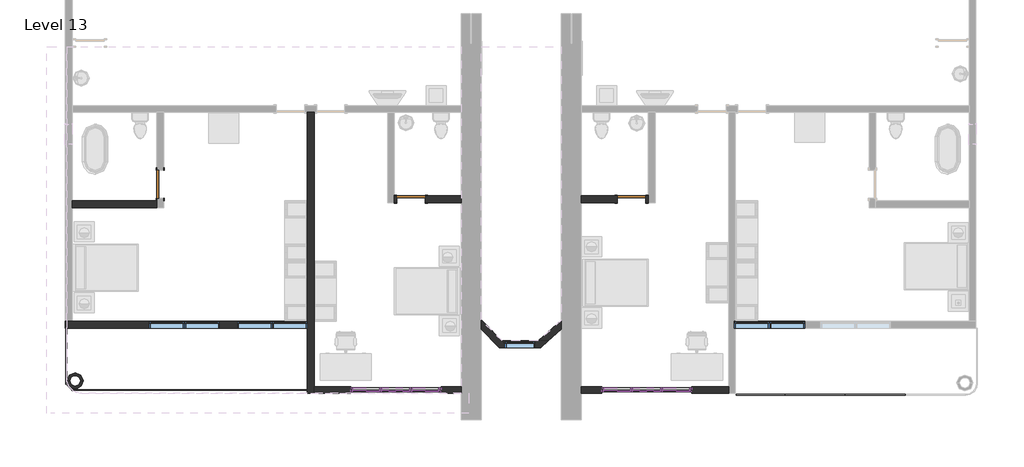
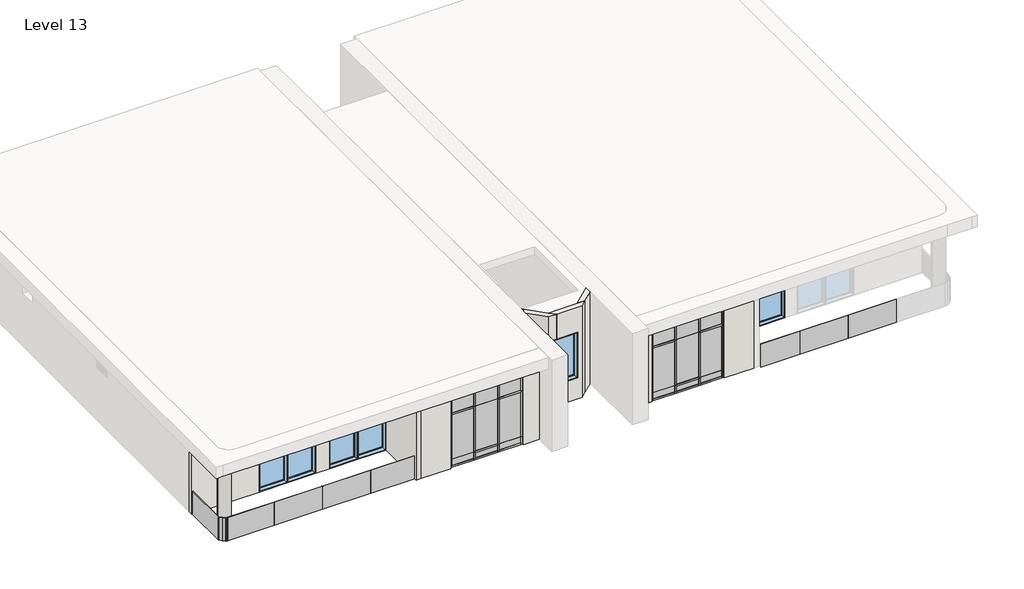
# One storey, part 1 of 3: 42 members, 30 plates, 14 walls, 7 windows, 3 doors.
"""IFC4 building model written with IfcOpenShell, lengths in millimetres."""

from ifc_helpers import new_model, si_unit, point, frame, frame_2d, origin, place, context, project, spatial, polyline, circle_curve, trimmed, segment, composite_curve, outline, extrude, faceted_brep, transform, mapped, element, save
from components import door_2703ae13, door_10fd3a06, member_c17f1be2, member_ad567e07, member_d2e7e466, member_7db1855a, member_75d1e245, member_d60e8053, member_3c3dc66a, member_2fae0574, member_410c6227, member_73c23c35, system_panel_glazed_38d54ecf, system_panel_glazed_fbb6c980, system_panel_glazed_4137532c, system_panel_glazed_6230de04, system_panel_glazed_a79f7f85, system_panel_glazed_9a5ea490, system_panel_glazed_95be5de7, system_panel_glazed_1e00a1c5, system_panel_glazed_ffe51582, system_panel_glazed_8f95e3f6, system_panel_glazed_836907cd, system_panel_glazed_688a65a2, system_panel_glazed_c1a1c740, system_panel_glazed_22bcd51f, window_9a779fa2, window_1a213a25

model = new_model("IFC4")

# Units and contexts
model_context = context("Model", 3, world=origin())
ifc_project = project(units=[si_unit("LENGTHUNIT", "METRE", prefix="MILLI")], contexts=[model_context])

# Site, building, storey
site = spatial("IfcSite", under=ifc_project)
building = spatial("IfcBuilding", under=site)
storey = spatial("IfcBuildingStorey", under=building, Name="Level 13", Elevation=43891.2)

# Doors
placement = place(None, origin())
door_shape = door_2703ae13(model_context)
element("IfcDoor", 1, ObjectType="Door-Single-Panel.0001 : 34\" x 80\"", at=placement, inside=storey, context=model_context, shape_type="MappedRepresentation", body=[
    mapped(door_shape, transform((-15765.9987704, -441.9241442, 43891.2), x_axis=(0.0, -1.0, 0.0), y_axis=(1.0, 0.0, 0.0), z_axis=(0.0, 0.0, 1.0))),
])
element("IfcDoor", 2, ObjectType="Door-Single-Panel.0001 : 34\" x 80\"", at=placement, inside=storey, context=model_context, shape_type="MappedRepresentation", body=[
    mapped(door_shape, transform((-8145.9987704, -899.1241442, 43891.2), x_axis=(-1.0, 0.0, 0.0), y_axis=(0.0, -1.0, 0.0), z_axis=(0.0, 0.0, 1.0))),
])
door_2_shape = door_10fd3a06(model_context)
element("IfcDoor", 3, ObjectType="Door-Single-Panel.0001 : 34\" x 80\"", at=placement, inside=storey, context=model_context, shape_type="MappedRepresentation", body=[
    mapped(door_2_shape, transform((-1440.3987704, -899.1241442, 43891.2), x_axis=(1.0, 0.0, 0.0), y_axis=(0.0, 1.0, 0.0), z_axis=(0.0, 0.0, 1.0))),
])

# Members
member_shape = member_c17f1be2(model_context)
element("IfcMember", 4, ObjectType="Rectangular Mullion : 2.5\" x 5\" rectangular", at=placement, inside=storey, context=model_context, shape_type="MappedRepresentation", body=[
    mapped(member_shape, transform((-9911.2987704, -6690.3241442, 46939.2), x_axis=(0.0, 0.0, 1.0), y_axis=(0.0, 1.0, 0.0), z_axis=(-1.0, 0.0, 0.0))),
])
element("IfcMember", 5, ObjectType="Rectangular Mullion : 2.5\" x 5\" rectangular", at=placement, inside=storey, context=model_context, shape_type="MappedRepresentation", body=[
    mapped(member_shape, transform((-8114.2487704, -6690.3241442, 46939.2), x_axis=(0.0, 0.0, 1.0), y_axis=(0.0, 1.0, 0.0), z_axis=(-1.0, 0.0, 0.0))),
])
element("IfcMember", 6, ObjectType="Rectangular Mullion : 2.5\" x 5\" rectangular", at=placement, inside=storey, context=model_context, shape_type="MappedRepresentation", body=[
    mapped(member_shape, transform((-2291.2987704, -6690.3241442, 46939.2), x_axis=(0.0, 0.0, 1.0), y_axis=(0.0, 1.0, 0.0), z_axis=(-1.0, 0.0, 0.0))),
])
element("IfcMember", 7, ObjectType="Rectangular Mullion : 2.5\" x 5\" rectangular", at=placement, inside=storey, context=model_context, shape_type="MappedRepresentation", body=[
    mapped(member_shape, transform((-494.2487704, -6690.3241442, 46939.2), x_axis=(0.0, 0.0, 1.0), y_axis=(0.0, 1.0, 0.0), z_axis=(-1.0, 0.0, 0.0))),
])
element("IfcMember", 8, ObjectType="Rectangular Mullion : 2.5\" x 5\" rectangular", at=placement, inside=storey, context=model_context, shape_type="MappedRepresentation", body=[
    mapped(member_shape, transform((-7295.0987704, -6690.3241442, 43891.2), x_axis=(0.0, 0.0, -1.0), y_axis=(0.0, 1.0, 0.0), z_axis=(1.0, 0.0, 0.0))),
])
element("IfcMember", 9, ObjectType="Rectangular Mullion : 2.5\" x 5\" rectangular", at=placement, inside=storey, context=model_context, shape_type="MappedRepresentation", body=[
    mapped(member_shape, transform((-9092.1487704, -6690.3241442, 43891.2), x_axis=(0.0, 0.0, -1.0), y_axis=(0.0, 1.0, 0.0), z_axis=(1.0, 0.0, 0.0))),
])
element("IfcMember", 10, ObjectType="Rectangular Mullion : 2.5\" x 5\" rectangular", at=placement, inside=storey, context=model_context, shape_type="MappedRepresentation", body=[
    mapped(member_shape, transform((324.9012296, -6690.3241442, 43891.2), x_axis=(0.0, 0.0, -1.0), y_axis=(0.0, 1.0, 0.0), z_axis=(1.0, 0.0, 0.0))),
])
element("IfcMember", 11, ObjectType="Rectangular Mullion : 2.5\" x 5\" rectangular", at=placement, inside=storey, context=model_context, shape_type="MappedRepresentation", body=[
    mapped(member_shape, transform((-1472.1487704, -6690.3241442, 43891.2), x_axis=(0.0, 0.0, -1.0), y_axis=(0.0, 1.0, 0.0), z_axis=(1.0, 0.0, 0.0))),
])
member_2_shape = member_ad567e07(model_context)
element("IfcMember", 12, ObjectType="Rectangular Mullion : 2.5\" x 5\" rectangular", at=placement, inside=storey, context=model_context, shape_type="MappedRepresentation", body=[
    mapped(member_2_shape, transform((-8114.2487704, -6690.3241442, 46024.8), x_axis=(0.0, 0.0, 1.0), y_axis=(0.0, 1.0, 0.0), z_axis=(-1.0, 0.0, 0.0))),
])
element("IfcMember", 13, ObjectType="Rectangular Mullion : 2.5\" x 5\" rectangular", at=placement, inside=storey, context=model_context, shape_type="MappedRepresentation", body=[
    mapped(member_2_shape, transform((-9911.2987704, -6690.3241442, 46024.8), x_axis=(0.0, 0.0, 1.0), y_axis=(0.0, 1.0, 0.0), z_axis=(-1.0, 0.0, 0.0))),
])
element("IfcMember", 14, ObjectType="Rectangular Mullion : 2.5\" x 5\" rectangular", at=placement, inside=storey, context=model_context, shape_type="MappedRepresentation", body=[
    mapped(member_2_shape, transform((-494.2487704, -6690.3241442, 46024.8), x_axis=(0.0, 0.0, 1.0), y_axis=(0.0, 1.0, 0.0), z_axis=(-1.0, 0.0, 0.0))),
])
element("IfcMember", 15, ObjectType="Rectangular Mullion : 2.5\" x 5\" rectangular", at=placement, inside=storey, context=model_context, shape_type="MappedRepresentation", body=[
    mapped(member_2_shape, transform((-2291.2987704, -6690.3241442, 46024.8), x_axis=(0.0, 0.0, 1.0), y_axis=(0.0, 1.0, 0.0), z_axis=(-1.0, 0.0, 0.0))),
])
member_3_shape = member_d2e7e466(model_context)
element("IfcMember", 16, ObjectType="Rectangular Mullion : 2.5\" x 5\" rectangular", at=placement, inside=storey, context=model_context, shape_type="MappedRepresentation", body=[
    mapped(member_3_shape, transform((-8177.7487704, -6690.3241442, 43891.2), x_axis=(0.0, 0.0, -1.0), y_axis=(0.0, 1.0, 0.0), z_axis=(1.0, 0.0, 0.0))),
])
element("IfcMember", 17, ObjectType="Rectangular Mullion : 2.5\" x 5\" rectangular", at=placement, inside=storey, context=model_context, shape_type="MappedRepresentation", body=[
    mapped(member_3_shape, transform((-557.7487704, -6690.3241442, 43891.2), x_axis=(0.0, 0.0, -1.0), y_axis=(0.0, 1.0, 0.0), z_axis=(1.0, 0.0, 0.0))),
])
member_4_shape = member_7db1855a(model_context)
element("IfcMember", 18, ObjectType="Rectangular Mullion : 2.5\" x 5\" rectangular", at=placement, inside=storey, context=model_context, shape_type="MappedRepresentation", body=[
    mapped(member_4_shape, transform((-9028.6487704, -6690.3241442, 44196.0), x_axis=(0.0, 0.0, 1.0), y_axis=(0.0, 1.0, 0.0), z_axis=(-1.0, 0.0, 0.0))),
])
element("IfcMember", 19, ObjectType="Rectangular Mullion : 2.5\" x 5\" rectangular", at=placement, inside=storey, context=model_context, shape_type="MappedRepresentation", body=[
    mapped(member_4_shape, transform((-1408.6487704, -6690.3241442, 44196.0), x_axis=(0.0, 0.0, 1.0), y_axis=(0.0, 1.0, 0.0), z_axis=(-1.0, 0.0, 0.0))),
])
element("IfcMember", 20, ObjectType="Rectangular Mullion : 2.5\" x 5\" rectangular", at=placement, inside=storey, context=model_context, shape_type="MappedRepresentation", body=[
    mapped(member_3_shape, transform((-9028.6487704, -6690.3241442, 46939.2), x_axis=(0.0, 0.0, 1.0), y_axis=(0.0, 1.0, 0.0), z_axis=(-1.0, 0.0, 0.0))),
])
element("IfcMember", 21, ObjectType="Rectangular Mullion : 2.5\" x 5\" rectangular", at=placement, inside=storey, context=model_context, shape_type="MappedRepresentation", body=[
    mapped(member_3_shape, transform((-1408.6487704, -6690.3241442, 46939.2), x_axis=(0.0, 0.0, 1.0), y_axis=(0.0, 1.0, 0.0), z_axis=(-1.0, 0.0, 0.0))),
])
member_5_shape = member_75d1e245(model_context)
element("IfcMember", 22, ObjectType="Rectangular Mullion : 2.5\" x 5\" rectangular", at=placement, inside=storey, context=model_context, shape_type="MappedRepresentation", body=[
    mapped(member_5_shape, transform((-8145.9987704, -6690.3241442, 43891.2), x_axis=(-1.0, 0.0, 0.0), y_axis=(0.0, 1.0, 0.0), z_axis=(0.0, 0.0, -1.0))),
])
element("IfcMember", 23, ObjectType="Rectangular Mullion : 2.5\" x 5\" rectangular", at=placement, inside=storey, context=model_context, shape_type="MappedRepresentation", body=[
    mapped(member_5_shape, transform((-9060.3987704, -6690.3241442, 43891.2), x_axis=(-1.0, 0.0, 0.0), y_axis=(0.0, 1.0, 0.0), z_axis=(0.0, 0.0, -1.0))),
])
element("IfcMember", 24, ObjectType="Rectangular Mullion : 2.5\" x 5\" rectangular", at=placement, inside=storey, context=model_context, shape_type="MappedRepresentation", body=[
    mapped(member_5_shape, transform((-525.9987704, -6690.3241442, 43891.2), x_axis=(-1.0, 0.0, 0.0), y_axis=(0.0, 1.0, 0.0), z_axis=(0.0, 0.0, -1.0))),
])
element("IfcMember", 25, ObjectType="Rectangular Mullion : 2.5\" x 5\" rectangular", at=placement, inside=storey, context=model_context, shape_type="MappedRepresentation", body=[
    mapped(member_5_shape, transform((-1440.3987704, -6690.3241442, 43891.2), x_axis=(-1.0, 0.0, 0.0), y_axis=(0.0, 1.0, 0.0), z_axis=(0.0, 0.0, -1.0))),
])
member_6_shape = member_d60e8053(model_context)
element("IfcMember", 26, ObjectType="Rectangular Mullion : 2.5\" x 5\" rectangular", at=placement, inside=storey, context=model_context, shape_type="MappedRepresentation", body=[
    mapped(member_6_shape, transform((-8145.9987704, -6690.3241442, 44196.0), x_axis=(-1.0, 0.0, 0.0), y_axis=(0.0, 1.0, 0.0), z_axis=(0.0, 0.0, -1.0))),
])
element("IfcMember", 27, ObjectType="Rectangular Mullion : 2.5\" x 5\" rectangular", at=placement, inside=storey, context=model_context, shape_type="MappedRepresentation", body=[
    mapped(member_6_shape, transform((-9060.3987704, -6690.3241442, 44196.0), x_axis=(-1.0, 0.0, 0.0), y_axis=(0.0, 1.0, 0.0), z_axis=(0.0, 0.0, -1.0))),
])
element("IfcMember", 28, ObjectType="Rectangular Mullion : 2.5\" x 5\" rectangular", at=placement, inside=storey, context=model_context, shape_type="MappedRepresentation", body=[
    mapped(member_6_shape, transform((-525.9987704, -6690.3241442, 44196.0), x_axis=(-1.0, 0.0, 0.0), y_axis=(0.0, 1.0, 0.0), z_axis=(0.0, 0.0, -1.0))),
])
element("IfcMember", 29, ObjectType="Rectangular Mullion : 2.5\" x 5\" rectangular", at=placement, inside=storey, context=model_context, shape_type="MappedRepresentation", body=[
    mapped(member_6_shape, transform((-1440.3987704, -6690.3241442, 44196.0), x_axis=(-1.0, 0.0, 0.0), y_axis=(0.0, 1.0, 0.0), z_axis=(0.0, 0.0, -1.0))),
])
member_7_shape = member_3c3dc66a(model_context)
element("IfcMember", 30, ObjectType="Rectangular Mullion : 2.5\" x 5\" rectangular", at=placement, inside=storey, context=model_context, shape_type="MappedRepresentation", body=[
    mapped(member_7_shape, transform((-9974.7987704, -6690.3241442, 43891.2), x_axis=(-1.0, 0.0, 0.0), y_axis=(0.0, 1.0, 0.0), z_axis=(0.0, 0.0, -1.0))),
])
element("IfcMember", 31, ObjectType="Rectangular Mullion : 2.5\" x 5\" rectangular", at=placement, inside=storey, context=model_context, shape_type="MappedRepresentation", body=[
    mapped(member_7_shape, transform((-2354.7987704, -6690.3241442, 43891.2), x_axis=(-1.0, 0.0, 0.0), y_axis=(0.0, 1.0, 0.0), z_axis=(0.0, 0.0, -1.0))),
])
member_8_shape = member_2fae0574(model_context)
element("IfcMember", 32, ObjectType="Rectangular Mullion : 2.5\" x 5\" rectangular", at=placement, inside=storey, context=model_context, shape_type="MappedRepresentation", body=[
    mapped(member_8_shape, transform((-9974.7987704, -6690.3241442, 44196.0), x_axis=(-1.0, 0.0, 0.0), y_axis=(0.0, 1.0, 0.0), z_axis=(0.0, 0.0, -1.0))),
])
element("IfcMember", 33, ObjectType="Rectangular Mullion : 2.5\" x 5\" rectangular", at=placement, inside=storey, context=model_context, shape_type="MappedRepresentation", body=[
    mapped(member_8_shape, transform((-2354.7987704, -6690.3241442, 44196.0), x_axis=(-1.0, 0.0, 0.0), y_axis=(0.0, 1.0, 0.0), z_axis=(0.0, 0.0, -1.0))),
])
element("IfcMember", 34, ObjectType="Rectangular Mullion : 2.5\" x 5\" rectangular", at=placement, inside=storey, context=model_context, shape_type="MappedRepresentation", body=[
    mapped(member_8_shape, transform((-7231.5987704, -6690.3241442, 46024.8), x_axis=(1.0, 0.0, 0.0), y_axis=(0.0, 1.0, 0.0), z_axis=(0.0, 0.0, 1.0))),
])
element("IfcMember", 35, ObjectType="Rectangular Mullion : 2.5\" x 5\" rectangular", at=placement, inside=storey, context=model_context, shape_type="MappedRepresentation", body=[
    mapped(member_8_shape, transform((388.4012296, -6690.3241442, 46024.8), x_axis=(1.0, 0.0, 0.0), y_axis=(0.0, 1.0, 0.0), z_axis=(0.0, 0.0, 1.0))),
])
element("IfcMember", 36, ObjectType="Rectangular Mullion : 2.5\" x 5\" rectangular", at=placement, inside=storey, context=model_context, shape_type="MappedRepresentation", body=[
    mapped(member_7_shape, transform((-7231.5987704, -6690.3241442, 44196.0), x_axis=(1.0, 0.0, 0.0), y_axis=(0.0, 1.0, 0.0), z_axis=(0.0, 0.0, 1.0))),
])
element("IfcMember", 37, ObjectType="Rectangular Mullion : 2.5\" x 5\" rectangular", at=placement, inside=storey, context=model_context, shape_type="MappedRepresentation", body=[
    mapped(member_7_shape, transform((388.4012296, -6690.3241442, 44196.0), x_axis=(1.0, 0.0, 0.0), y_axis=(0.0, 1.0, 0.0), z_axis=(0.0, 0.0, 1.0))),
])
member_9_shape = member_410c6227(model_context)
element("IfcMember", 38, ObjectType="Rectangular Mullion : 2.5\" x 5\" rectangular", at=placement, inside=storey, context=model_context, shape_type="MappedRepresentation", body=[
    mapped(member_9_shape, transform((-8145.9987704, -6690.3241442, 46024.8), x_axis=(-1.0, 0.0, 0.0), y_axis=(0.0, 1.0, 0.0), z_axis=(0.0, 0.0, -1.0))),
])
element("IfcMember", 39, ObjectType="Rectangular Mullion : 2.5\" x 5\" rectangular", at=placement, inside=storey, context=model_context, shape_type="MappedRepresentation", body=[
    mapped(member_9_shape, transform((-9060.3987704, -6690.3241442, 46024.8), x_axis=(-1.0, 0.0, 0.0), y_axis=(0.0, 1.0, 0.0), z_axis=(0.0, 0.0, -1.0))),
])
element("IfcMember", 40, ObjectType="Rectangular Mullion : 2.5\" x 5\" rectangular", at=placement, inside=storey, context=model_context, shape_type="MappedRepresentation", body=[
    mapped(member_9_shape, transform((-525.9987704, -6690.3241442, 46024.8), x_axis=(-1.0, 0.0, 0.0), y_axis=(0.0, 1.0, 0.0), z_axis=(0.0, 0.0, -1.0))),
])
element("IfcMember", 41, ObjectType="Rectangular Mullion : 2.5\" x 5\" rectangular", at=placement, inside=storey, context=model_context, shape_type="MappedRepresentation", body=[
    mapped(member_9_shape, transform((-1440.3987704, -6690.3241442, 46024.8), x_axis=(-1.0, 0.0, 0.0), y_axis=(0.0, 1.0, 0.0), z_axis=(0.0, 0.0, -1.0))),
])
member_10_shape = member_73c23c35(model_context)
element("IfcMember", 42, ObjectType="Rectangular Mullion : 2.5\" x 5\" rectangular", at=placement, inside=storey, context=model_context, shape_type="MappedRepresentation", body=[
    mapped(member_10_shape, transform((-7231.5987704, -6690.3241442, 46939.2), x_axis=(1.0, 0.0, 0.0), y_axis=(0.0, 1.0, 0.0), z_axis=(0.0, 0.0, 1.0))),
])
element("IfcMember", 43, ObjectType="Rectangular Mullion : 2.5\" x 5\" rectangular", at=placement, inside=storey, context=model_context, shape_type="MappedRepresentation", body=[
    mapped(member_10_shape, transform((388.4012296, -6690.3241442, 46939.2), x_axis=(1.0, 0.0, 0.0), y_axis=(0.0, 1.0, 0.0), z_axis=(0.0, 0.0, 1.0))),
])
element("IfcMember", 44, ObjectType="Rectangular Mullion : 2.5\" x 5\" rectangular", at=placement, inside=storey, context=model_context, shape_type="MappedRepresentation", body=[
    mapped(member_10_shape, transform((-9974.7987704, -6690.3241442, 46024.8), x_axis=(-1.0, 0.0, 0.0), y_axis=(0.0, 1.0, 0.0), z_axis=(0.0, 0.0, -1.0))),
])
element("IfcMember", 45, ObjectType="Rectangular Mullion : 2.5\" x 5\" rectangular", at=placement, inside=storey, context=model_context, shape_type="MappedRepresentation", body=[
    mapped(member_10_shape, transform((-2354.7987704, -6690.3241442, 46024.8), x_axis=(-1.0, 0.0, 0.0), y_axis=(0.0, 1.0, 0.0), z_axis=(0.0, 0.0, -1.0))),
])

# Plates
system_panel_glazed_shape = system_panel_glazed_38d54ecf(model_context)
element("IfcPlate", 46, ObjectType="System Panel : Glazed", at=placement, inside=storey, context=model_context, shape_type="MappedRepresentation", body=[
    mapped(system_panel_glazed_shape, transform((-8603.1987704, -6690.3241442, 44227.75), x_axis=(-1.0, 0.0, 0.0), y_axis=(0.0, -1.0, 0.0), z_axis=(0.0, 0.0, 1.0))),
])
element("IfcPlate", 47, ObjectType="System Panel : Glazed", at=placement, inside=storey, context=model_context, shape_type="MappedRepresentation", body=[
    mapped(system_panel_glazed_shape, transform((-983.1987704, -6690.3241442, 44227.75), x_axis=(-1.0, 0.0, 0.0), y_axis=(0.0, -1.0, 0.0), z_axis=(0.0, 0.0, 1.0))),
])
system_panel_glazed_2_shape = system_panel_glazed_fbb6c980(model_context)
element("IfcPlate", 48, ObjectType="System Panel : Glazed", at=placement, inside=storey, context=model_context, shape_type="MappedRepresentation", body=[
    mapped(system_panel_glazed_2_shape, transform((-8603.1987704, -6690.3241442, 43954.7), x_axis=(-1.0, 0.0, 0.0), y_axis=(0.0, -1.0, 0.0), z_axis=(0.0, 0.0, 1.0))),
])
element("IfcPlate", 49, ObjectType="System Panel : Glazed", at=placement, inside=storey, context=model_context, shape_type="MappedRepresentation", body=[
    mapped(system_panel_glazed_2_shape, transform((-983.1987704, -6690.3241442, 43954.7), x_axis=(-1.0, 0.0, 0.0), y_axis=(0.0, -1.0, 0.0), z_axis=(0.0, 0.0, 1.0))),
])
system_panel_glazed_3_shape = system_panel_glazed_4137532c(model_context)
element("IfcPlate", 50, ObjectType="System Panel : Glazed", at=placement, inside=storey, context=model_context, shape_type="MappedRepresentation", body=[
    mapped(system_panel_glazed_3_shape, transform((-7704.6737704, -6690.3241442, 43954.7), x_axis=(-1.0, 0.0, 0.0), y_axis=(0.0, -1.0, 0.0), z_axis=(0.0, 0.0, 1.0))),
])
element("IfcPlate", 51, ObjectType="System Panel : Glazed", at=placement, inside=storey, context=model_context, shape_type="MappedRepresentation", body=[
    mapped(system_panel_glazed_3_shape, transform((-9501.7237704, -6690.3241442, 43954.7), x_axis=(-1.0, 0.0, 0.0), y_axis=(0.0, -1.0, 0.0), z_axis=(0.0, 0.0, 1.0))),
])
element("IfcPlate", 52, ObjectType="System Panel : Glazed", at=placement, inside=storey, context=model_context, shape_type="MappedRepresentation", body=[
    mapped(system_panel_glazed_3_shape, transform((-84.6737704, -6690.3241442, 43954.7), x_axis=(-1.0, 0.0, 0.0), y_axis=(0.0, -1.0, 0.0), z_axis=(0.0, 0.0, 1.0))),
])
element("IfcPlate", 53, ObjectType="System Panel : Glazed", at=placement, inside=storey, context=model_context, shape_type="MappedRepresentation", body=[
    mapped(system_panel_glazed_3_shape, transform((-1881.7237704, -6690.3241442, 43954.7), x_axis=(-1.0, 0.0, 0.0), y_axis=(0.0, -1.0, 0.0), z_axis=(0.0, 0.0, 1.0))),
])
system_panel_glazed_4_shape = system_panel_glazed_6230de04(model_context)
element("IfcPlate", 54, ObjectType="System Panel : Glazed", at=placement, inside=storey, context=model_context, shape_type="MappedRepresentation", body=[
    mapped(system_panel_glazed_4_shape, transform((-7704.6737704, -6690.3241442, 44196.0), x_axis=(-1.0, 0.0, 0.0), y_axis=(0.0, -1.0, 0.0), z_axis=(0.0, 0.0, 1.0))),
])
element("IfcPlate", 55, ObjectType="System Panel : Glazed", at=placement, inside=storey, context=model_context, shape_type="MappedRepresentation", body=[
    mapped(system_panel_glazed_4_shape, transform((-9501.7237704, -6690.3241442, 44196.0), x_axis=(-1.0, 0.0, 0.0), y_axis=(0.0, -1.0, 0.0), z_axis=(0.0, 0.0, 1.0))),
])
element("IfcPlate", 56, ObjectType="System Panel : Glazed", at=placement, inside=storey, context=model_context, shape_type="MappedRepresentation", body=[
    mapped(system_panel_glazed_4_shape, transform((-84.6737704, -6690.3241442, 44196.0), x_axis=(-1.0, 0.0, 0.0), y_axis=(0.0, -1.0, 0.0), z_axis=(0.0, 0.0, 1.0))),
])
element("IfcPlate", 57, ObjectType="System Panel : Glazed", at=placement, inside=storey, context=model_context, shape_type="MappedRepresentation", body=[
    mapped(system_panel_glazed_4_shape, transform((-1881.7237704, -6690.3241442, 44196.0), x_axis=(-1.0, 0.0, 0.0), y_axis=(0.0, -1.0, 0.0), z_axis=(0.0, 0.0, 1.0))),
])
system_panel_glazed_5_shape = system_panel_glazed_a79f7f85(model_context)
element("IfcPlate", 58, ObjectType="System Panel : Glazed", at=placement, inside=storey, context=model_context, shape_type="MappedRepresentation", body=[
    mapped(system_panel_glazed_5_shape, transform((-7704.6737704, -6690.3241442, 46056.55), x_axis=(-1.0, 0.0, 0.0), y_axis=(0.0, -1.0, 0.0), z_axis=(0.0, 0.0, 1.0))),
])
element("IfcPlate", 59, ObjectType="System Panel : Glazed", at=placement, inside=storey, context=model_context, shape_type="MappedRepresentation", body=[
    mapped(system_panel_glazed_5_shape, transform((-9501.7237704, -6690.3241442, 46056.55), x_axis=(-1.0, 0.0, 0.0), y_axis=(0.0, -1.0, 0.0), z_axis=(0.0, 0.0, 1.0))),
])
element("IfcPlate", 60, ObjectType="System Panel : Glazed", at=placement, inside=storey, context=model_context, shape_type="MappedRepresentation", body=[
    mapped(system_panel_glazed_5_shape, transform((-84.6737704, -6690.3241442, 46056.55), x_axis=(-1.0, 0.0, 0.0), y_axis=(0.0, -1.0, 0.0), z_axis=(0.0, 0.0, 1.0))),
])
element("IfcPlate", 61, ObjectType="System Panel : Glazed", at=placement, inside=storey, context=model_context, shape_type="MappedRepresentation", body=[
    mapped(system_panel_glazed_5_shape, transform((-1881.7237704, -6690.3241442, 46056.55), x_axis=(-1.0, 0.0, 0.0), y_axis=(0.0, -1.0, 0.0), z_axis=(0.0, 0.0, 1.0))),
])
system_panel_glazed_6_shape = system_panel_glazed_9a5ea490(model_context)
element("IfcPlate", 62, ObjectType="System Panel : Glazed", at=placement, inside=storey, context=model_context, shape_type="MappedRepresentation", body=[
    mapped(system_panel_glazed_6_shape, transform((-8603.1987704, -6690.3241442, 46024.8), x_axis=(-1.0, 0.0, 0.0), y_axis=(0.0, -1.0, 0.0), z_axis=(0.0, 0.0, 1.0))),
])
element("IfcPlate", 63, ObjectType="System Panel : Glazed", at=placement, inside=storey, context=model_context, shape_type="MappedRepresentation", body=[
    mapped(system_panel_glazed_6_shape, transform((-983.1987704, -6690.3241442, 46024.8), x_axis=(-1.0, 0.0, 0.0), y_axis=(0.0, -1.0, 0.0), z_axis=(0.0, 0.0, 1.0))),
])
system_panel_glazed_7_shape = system_panel_glazed_95be5de7(model_context)
element("IfcPlate", 64, ObjectType="System Panel : Glazed", at=placement, inside=storey, context=model_context, shape_type="MappedRepresentation", body=[
    mapped(system_panel_glazed_7_shape, transform((-15707.2305745, -6723.6923401, 43891.2), x_axis=(1.0, 0.0, 0.0), y_axis=(0.0, 1.0, 0.0), z_axis=(0.0, 0.0, 1.0))),
])
element("IfcPlate", 65, ObjectType="System Panel : Glazed", at=placement, inside=storey, context=model_context, shape_type="MappedRepresentation", body=[
    mapped(system_panel_glazed_7_shape, transform((-13878.4305745, -6723.6923401, 43891.2), x_axis=(1.0, 0.0, 0.0), y_axis=(0.0, 1.0, 0.0), z_axis=(0.0, 0.0, 1.0))),
])
element("IfcPlate", 66, ObjectType="System Panel : Glazed", at=placement, inside=storey, context=model_context, shape_type="MappedRepresentation", body=[
    mapped(system_panel_glazed_7_shape, transform((5957.9120092, -6810.4133646, 43891.2), x_axis=(-1.0, 0.0, 0.0), y_axis=(0.0, -1.0, 0.0), z_axis=(0.0, 0.0, 1.0))),
])
element("IfcPlate", 67, ObjectType="System Panel : Glazed", at=placement, inside=storey, context=model_context, shape_type="MappedRepresentation", body=[
    mapped(system_panel_glazed_7_shape, transform((4129.1120092, -6810.4133646, 43891.2), x_axis=(-1.0, 0.0, 0.0), y_axis=(0.0, -1.0, 0.0), z_axis=(0.0, 0.0, 1.0))),
])
system_panel_glazed_8_shape = system_panel_glazed_1e00a1c5(model_context)
element("IfcPlate", 68, ObjectType="System Panel : Glazed", at=placement, inside=storey, context=model_context, shape_type="MappedRepresentation", body=[
    mapped(system_panel_glazed_8_shape, transform((2478.1120092, -6810.4133646, 43891.2), x_axis=(-1.0, 0.0, 0.0), y_axis=(0.0, -1.0, 0.0), z_axis=(0.0, 0.0, 1.0))),
])
system_panel_glazed_9_shape = system_panel_glazed_ffe51582(model_context)
element("IfcPlate", 69, ObjectType="System Panel : Glazed", at=placement, inside=storey, context=model_context, shape_type="MappedRepresentation", body=[
    mapped(system_panel_glazed_9_shape, transform((-18451.9713429, -6722.1515718, 43891.2), x_axis=(0.7071067811865462, -0.7071067811865488, 0.0), y_axis=(0.7071067811865488, 0.7071067811865462, 0.0), z_axis=(0.0, 0.0, 1.0))),
])
system_panel_glazed_10_shape = system_panel_glazed_8f95e3f6(model_context)
element("IfcPlate", 70, ObjectType="System Panel : Glazed", at=placement, inside=storey, context=model_context, shape_type="MappedRepresentation", body=[
    mapped(system_panel_glazed_10_shape, transform((-18648.8987704, -5667.9741442, 43891.2), x_axis=(0.0, -1.0, 0.0), y_axis=(1.0, 0.0, 0.0), z_axis=(0.0, 0.0, 1.0))),
])
system_panel_glazed_11_shape = system_panel_glazed_836907cd(model_context)
element("IfcPlate", 71, ObjectType="System Panel : Glazed", at=placement, inside=storey, context=model_context, shape_type="MappedRepresentation", body=[
    mapped(system_panel_glazed_11_shape, transform((-18418.6805745, -6723.6923401, 43891.2), x_axis=(1.0, 0.0, 0.0), y_axis=(0.0, 1.0, 0.0), z_axis=(0.0, 0.0, 1.0))),
])
system_panel_glazed_12_shape = system_panel_glazed_688a65a2(model_context)
element("IfcPlate", 72, ObjectType="System Panel : Glazed", at=placement, inside=storey, context=model_context, shape_type="MappedRepresentation", body=[
    mapped(system_panel_glazed_12_shape, transform((-12129.8146725, -6723.6923401, 43891.2), x_axis=(1.0, 0.0, 0.0), y_axis=(0.0, 1.0, 0.0), z_axis=(0.0, 0.0, 1.0))),
])
system_panel_glazed_13_shape = system_panel_glazed_c1a1c740(model_context)
element("IfcPlate", 73, ObjectType="System Panel : Glazed", at=placement, inside=storey, context=model_context, shape_type="MappedRepresentation", body=[
    mapped(system_panel_glazed_13_shape, transform((-17504.2805745, -6723.6923401, 43891.2), x_axis=(1.0, 0.0, 0.0), y_axis=(0.0, 1.0, 0.0), z_axis=(0.0, 0.0, 1.0))),
])
system_panel_glazed_14_shape = system_panel_glazed_22bcd51f(model_context)
element("IfcPlate", 74, ObjectType="System Panel : Glazed", at=placement, inside=storey, context=model_context, shape_type="MappedRepresentation", body=[
    mapped(system_panel_glazed_14_shape, transform((-18600.0521056, -6574.070809, 43891.2), x_axis=(0.7071067811865462, -0.7071067811865488, 0.0), y_axis=(0.7071067811865488, 0.7071067811865462, 0.0), z_axis=(0.0, 0.0, 1.0))),
])
element("IfcPlate", 75, ObjectType="System Panel : Glazed", at=placement, inside=storey, context=model_context, shape_type="MappedRepresentation", body=[
    mapped(system_panel_glazed_14_shape, transform((-18502.3587761, -6671.7641386, 43891.2), x_axis=(0.7071067811865462, -0.7071067811865488, 0.0), y_axis=(0.7071067811865488, 0.7071067811865462, 0.0), z_axis=(0.0, 0.0, 1.0))),
])

# Walls
element("IfcWall", 76, ObjectType="Generic - 3\" green 2", at=placement, inside=storey, context=model_context, shape_type="SweptSolid", body=[
    extrude(outline(composite_curve([segment(polyline([(-18518.7237704, -6418.8616442), (-18594.9237704, -6418.8616442)]), True, "CONTINUOUS"), segment(trimmed(circle_curve(frame_2d((-18353.6237704, -6418.8616442)), 241.3), [point((-18594.9237704, -6418.8616442))], [point((-18112.3237704, -6418.8616442))], False, "CARTESIAN"), True, "CONTINUOUS"), segment(polyline([(-18112.3237704, -6418.8616442), (-18188.5237704, -6418.8616442)]), True, "CONTINUOUS"), segment(trimmed(circle_curve(frame_2d((-18353.6237704, -6418.8616442)), 165.1), [point((-18188.5237704, -6418.8616442))], [point((-18518.7237704, -6418.8616442))], True, "CARTESIAN"), True, "CONTINUOUS")], self_intersect=False)), frame((0.0, 0.0, 43891.2), z_axis=(0.0, 0.0, 1.0), x_axis=(1.0, 0.0, 0.0)), (0.0, 0.0, 1.0), 3048.0),
])
element("IfcWall", 77, ObjectType="Generic - 3\" green 2", at=placement, inside=storey, context=model_context, shape_type="SweptSolid", body=[
    extrude(outline(composite_curve([segment(polyline([(-18188.5237704, -6418.8616442), (-18112.3237704, -6418.8616442)]), True, "CONTINUOUS"), segment(trimmed(circle_curve(frame_2d((-18353.6237704, -6418.8616442)), 241.3), [point((-18112.3237704, -6418.8616442))], [point((-18594.9237704, -6418.8616442))], False, "CARTESIAN"), True, "CONTINUOUS"), segment(polyline([(-18594.9237704, -6418.8616442), (-18518.7237704, -6418.8616442)]), True, "CONTINUOUS"), segment(trimmed(circle_curve(frame_2d((-18353.6237704, -6418.8616442)), 165.1), [point((-18518.7237704, -6418.8616442))], [point((-18188.5237704, -6418.8616442))], True, "CARTESIAN"), True, "CONTINUOUS")], self_intersect=False)), frame((0.0, 0.0, 43891.2), z_axis=(0.0, 0.0, 1.0), x_axis=(1.0, 0.0, 0.0)), (0.0, 0.0, 1.0), 3048.0),
])
element("IfcWall", 78, ObjectType="Generic - 8\" cream", at=placement, inside=storey, context=model_context, shape_type="Brep", body=[
    faceted_brep([(-11295.5987704, 1742.4758558, 43891.2), (-11295.5987704, -6791.9241442, 43891.2), (-11295.5987704, -6791.9241442, 46939.2), (-11295.5987704, -4810.7241442, 46939.2), (-11295.5987704, -4607.5241442, 46939.2), (-11295.5987704, 1742.4758558, 46939.2), (-11092.3987704, 1742.4758558, 43891.2), (-11092.3987704, 1742.4758558, 46939.2), (-11092.3987704, -6588.7241442, 46939.2), (-11092.3987704, -6791.9241442, 46939.2), (-11092.3987704, -6791.9241442, 43891.2), (-11092.3987704, -6588.7241442, 43891.2)], [[[0, 1, 2, 3, 4, 5]], [[6, 7, 8, 9, 10, 11]], [[1, 0, 6, 11, 10]], [[5, 4, 3, 2, 9, 8, 7]], [[0, 5, 7, 6]], [[2, 1, 10, 9]]]),
])
element("IfcWall", 79, ObjectType="Generic - 8\" cream", at=placement, inside=storey, context=model_context, shape_type="SweptSolid", body=[
    extrude(outline(polyline([(-18445.6987704, -949.9241442), (-15867.5987704, -949.9241442), (-15867.5987704, -1153.1241442), (-18445.6987704, -1153.1241442), (-18445.6987704, -949.9241442)])), frame((0.0, 0.0, 43891.2), z_axis=(0.0, 0.0, 1.0), x_axis=(1.0, 0.0, 0.0)), (0.0, 0.0, 1.0), 3048.0),
])
element("IfcWall", 80, ObjectType="Generic - 8\" cream", at=placement, inside=storey, context=model_context, shape_type="SweptSolid", body=[
    extrude(outline(polyline([(46939.2, -6621.9987704), (46939.2, -8653.9987704), (43891.2, -8653.9987704), (43891.2, -8577.7987704), (45923.2, -8577.7987704), (45923.2, -7714.1987704), (43891.2, -7714.1987704), (43891.2, -6621.9987704), (46939.2, -6621.9987704)])), frame((0.0, -1000.7241442, 0.0), z_axis=(0.0, 1.0, 0.0), x_axis=(0.0, 0.0, 1.0)), (0.0, 0.0, 1.0), 203.2),
])
element("IfcWall", 81, ObjectType="Generic - 8\" cream", at=placement, inside=storey, context=model_context, shape_type="Brep", body=[
    faceted_brep([(-18648.8987704, -4607.5241442, 46939.2), (-18445.6987704, -4607.5241442, 46939.2), (-11295.5987704, -4607.5241442, 46939.2), (-11295.5987704, -4607.5241442, 46634.4), (-13429.1987704, -4607.5241442, 46634.4), (-13429.1987704, -4607.5241442, 43891.2), (-13962.5987704, -4607.5241442, 43891.2), (-13962.5987704, -4607.5241442, 46634.4), (-16096.1987704, -4607.5241442, 46634.4), (-16096.1987704, -4607.5241442, 43891.2), (-18445.6987704, -4607.5241442, 43891.2), (-18648.8987704, -4607.5241442, 43891.2), (-11295.5987704, -4810.7241442, 46939.2), (-18648.8987704, -4810.7241442, 46939.2), (-18648.8987704, -4810.7241442, 43891.2), (-16096.1987704, -4810.7241442, 43891.2), (-16096.1987704, -4810.7241442, 46634.4), (-13962.5987704, -4810.7241442, 46634.4), (-13962.5987704, -4810.7241442, 43891.2), (-13429.1987704, -4810.7241442, 43891.2), (-13429.1987704, -4810.7241442, 46634.4), (-11295.5987704, -4810.7241442, 46634.4)], [[[0, 1, 2, 3, 4, 5, 6, 7, 8, 9, 10, 11]], [[12, 13, 14, 15, 16, 17, 18, 19, 20, 21]], [[14, 11, 10, 9, 15]], [[5, 19, 18, 6]], [[2, 1, 0, 13, 12]], [[2, 12, 21, 3]], [[0, 11, 14, 13]], [[3, 21, 20, 4]], [[4, 20, 19, 5]], [[17, 7, 6, 18]], [[7, 17, 16, 8]], [[8, 16, 15, 9]]]),
])
element("IfcWall", 82, ObjectType="Generic - 8\" cream", at=placement, inside=storey, context=model_context, shape_type="SweptSolid", body=[
    extrude(outline(polyline([(46939.2, -932.3987704), (46939.2, -2964.3987704), (43891.2, -2964.3987704), (43891.2, -1872.1987704), (45923.2, -1872.1987704), (45923.2, -1008.5987704), (43891.2, -1008.5987704), (43891.2, -932.3987704), (46939.2, -932.3987704)])), frame((0.0, -1000.7241442, 0.0), z_axis=(0.0, 1.0, 0.0), x_axis=(0.0, 0.0, 1.0)), (0.0, 0.0, 1.0), 203.2),
])
element("IfcWall", 83, ObjectType="Generic - 8\" cream", at=placement, inside=storey, context=model_context, shape_type="SweptSolid", body=[
    extrude(outline(polyline([(388.4012296, -6588.7241442), (1506.0012296, -6588.7241442), (1506.0012296, -6791.9241442), (388.4012296, -6791.9241442), (388.4012296, -6588.7241442)])), frame((0.0, 0.0, 43891.2), z_axis=(0.0, 0.0, 1.0), x_axis=(1.0, 0.0, 0.0)), (0.0, 0.0, 1.0), 3048.0),
])
element("IfcWall", 84, ObjectType="Generic - 8\" cream", at=placement, inside=storey, context=model_context, shape_type="SweptSolid", body=[
    extrude(outline(polyline([(-2354.7987704, -6791.9241442), (-2964.3987704, -6791.9241442), (-2964.3987704, -6588.7241442), (-2354.7987704, -6588.7241442), (-2354.7987704, -6791.9241442)])), frame((0.0, 0.0, 43891.2), z_axis=(0.0, 0.0, 1.0), x_axis=(1.0, 0.0, 0.0)), (0.0, 0.0, 1.0), 3048.0),
])
element("IfcWall", 85, ObjectType="Generic - 8\" cream", at=placement, inside=storey, context=model_context, shape_type="SweptSolid", body=[
    extrude(outline(polyline([(-9974.7987704, -6791.9241442), (-11092.3987704, -6791.9241442), (-11092.3987704, -6588.7241442), (-9974.7987704, -6588.7241442), (-9974.7987704, -6791.9241442)])), frame((0.0, 0.0, 43891.2), z_axis=(0.0, 0.0, 1.0), x_axis=(1.0, 0.0, 0.0)), (0.0, 0.0, 1.0), 3048.0),
])
element("IfcWall", 86, ObjectType="Generic - 8\" cream", at=placement, inside=storey, context=model_context, shape_type="SweptSolid", body=[
    extrude(outline(polyline([(-7231.5987704, -6588.7241442), (-6621.9987704, -6588.7241442), (-6621.9987704, -6791.9241442), (-7231.5987704, -6791.9241442), (-7231.5987704, -6588.7241442)])), frame((0.0, 0.0, 43891.2), z_axis=(0.0, 0.0, 1.0), x_axis=(1.0, 0.0, 0.0)), (0.0, 0.0, 1.0), 3048.0),
])
element("IfcWall", 87, ObjectType="Generic - 8\" green", at=placement, inside=storey, context=model_context, shape_type="Brep", body=[
    faceted_brep([(-6012.3987704, -4852.8082422, 43891.2), (-5458.7044276, -5406.502585, 43891.2), (-5458.7044276, -5406.502585, 47548.8), (-6012.3987704, -4852.8082422, 47548.8), (-5171.3362318, -5406.502585, 43891.2), (-5374.5362318, -5203.302585, 43891.2), (-6012.3987704, -4565.4400463, 43891.2), (-6012.3987704, -4565.4400463, 47548.8), (-5374.5362318, -5203.302585, 47548.8), (-5171.3362318, -5406.502585, 47548.8), (-5171.3362318, -5406.502585, 46558.2), (-5289.4901401, -5288.3486766, 46558.2), (-5289.4901401, -5288.3486766, 44729.4), (-5171.3362318, -5406.502585, 44729.4), (-5289.4901401, -5406.502585, 44729.4), (-5289.4901401, -5406.502585, 46558.2)], [[[0, 1, 2, 3]], [[4, 5, 6, 7, 8, 9, 10, 11, 12, 13]], [[1, 0, 6, 5, 4]], [[3, 2, 9, 8, 7]], [[0, 3, 7, 6]], [[2, 1, 4, 13, 14, 15, 10, 9]], [[12, 14, 13]], [[14, 12, 11, 15]], [[15, 11, 10]]]),
])
element("IfcWall", 88, ObjectType="Generic - 8\" green", at=placement, inside=storey, context=model_context, shape_type="Brep", body=[
    faceted_brep([(-5171.3362318, -5406.502585, 43891.2), (-4203.3343712, -5406.502585, 43891.2), (-4203.3343712, -5406.502585, 47548.8), (-5171.3362318, -5406.502585, 47548.8), (-5171.3362318, -5406.502585, 46558.2), (-4375.0901401, -5406.502585, 46558.2), (-4375.0901401, -5406.502585, 44729.4), (-5171.3362318, -5406.502585, 44729.4), (-3975.4820774, -5203.302585, 43891.2), (-4280.7801413, -5203.302585, 43891.2), (-5374.5362318, -5203.302585, 43891.2), (-5374.5362318, -5203.302585, 47548.8), (-4280.7801413, -5203.302585, 47548.8), (-3975.4820774, -5203.302585, 47548.8), (-4375.0901401, -5203.302585, 44729.4), (-4375.0901401, -5203.302585, 46558.2), (-5289.4901401, -5203.302585, 46558.2), (-5289.4901401, -5203.302585, 44729.4), (-5289.4901401, -5288.3486766, 44729.4), (-5289.4901401, -5288.3486766, 46558.2)], [[[0, 1, 2, 3, 4, 5, 6, 7]], [[8, 9, 10, 11, 12, 13], [14, 15, 16, 17]], [[1, 0, 10, 9, 8]], [[3, 2, 13, 12, 11]], [[3, 11, 10, 0, 7, 18, 19, 4]], [[2, 1, 8, 13]], [[5, 15, 14, 6]], [[6, 14, 17, 18, 7]], [[18, 17, 16, 19]], [[15, 5, 4, 19, 16]]]),
])
element("IfcWall", 89, ObjectType="Generic - 8\" green", at=placement, inside=storey, context=model_context, shape_type="SweptSolid", body=[
    extrude(outline(polyline([(-3573.9987704, -4845.2574382), (-3975.4820774, -5203.302585), (-4280.7801413, -5203.302585), (-3573.9987704, -4572.9908503), (-3573.9987704, -4845.2574382)])), frame((0.0, 0.0, 43891.2), z_axis=(0.0, 0.0, 1.0), x_axis=(1.0, 0.0, 0.0)), (0.0, 0.0, 1.0), 3657.6),
])

# Windows
window_shape = window_9a779fa2(model_context)
element("IfcWindow", 90, ObjectType="Fixed : 36\" x 72\"", at=placement, inside=storey, context=model_context, shape_type="MappedRepresentation", body=[
    mapped(window_shape, transform((-4794.1901401, -5304.902585, 44424.6), x_axis=(1.0, 0.0, 0.0), y_axis=(0.0, 1.0, 0.0), z_axis=(0.0, 0.0, 1.0))),
])
window_2_shape = window_1a213a25(model_context)
element("IfcWindow", 91, ObjectType="Fixed : 36\" x 72\" 2", at=placement, inside=storey, context=model_context, shape_type="MappedRepresentation", body=[
    mapped(window_2_shape, transform((-11790.8987704, -4709.1241442, 43586.4), x_axis=(1.0, 0.0, 0.0), y_axis=(0.0, 1.0, 0.0), z_axis=(0.0, 0.0, 1.0))),
])
element("IfcWindow", 92, ObjectType="Fixed : 36\" x 72\" 2", at=placement, inside=storey, context=model_context, shape_type="MappedRepresentation", body=[
    mapped(window_2_shape, transform((-12857.6987704, -4709.1241442, 43586.4), x_axis=(1.0, 0.0, 0.0), y_axis=(0.0, 1.0, 0.0), z_axis=(0.0, 0.0, 1.0))),
])
element("IfcWindow", 93, ObjectType="Fixed : 36\" x 72\" 2", at=placement, inside=storey, context=model_context, shape_type="MappedRepresentation", body=[
    mapped(window_2_shape, transform((-14457.8987704, -4709.1241442, 43586.4), x_axis=(1.0, 0.0, 0.0), y_axis=(0.0, 1.0, 0.0), z_axis=(0.0, 0.0, 1.0))),
])
element("IfcWindow", 94, ObjectType="Fixed : 36\" x 72\" 2", at=placement, inside=storey, context=model_context, shape_type="MappedRepresentation", body=[
    mapped(window_2_shape, transform((-15524.6987704, -4709.1241442, 43586.4), x_axis=(1.0, 0.0, 0.0), y_axis=(0.0, 1.0, 0.0), z_axis=(0.0, 0.0, 1.0))),
])
element("IfcWindow", 95, ObjectType="Fixed : 36\" x 72\" 2", at=placement, inside=storey, context=model_context, shape_type="MappedRepresentation", body=[
    mapped(window_2_shape, transform((2255.3012296, -4709.1241442, 43586.4), x_axis=(1.0, 0.0, 0.0), y_axis=(0.0, 1.0, 0.0), z_axis=(0.0, 0.0, 1.0))),
])
element("IfcWindow", 96, ObjectType="Fixed : 36\" x 72\" 2", at=placement, inside=storey, context=model_context, shape_type="MappedRepresentation", body=[
    mapped(window_2_shape, transform((3331.6262296, -4709.1241442, 43586.4), x_axis=(1.0, 0.0, 0.0), y_axis=(0.0, 1.0, 0.0), z_axis=(0.0, 0.0, 1.0))),
])

save(model, "model.ifc")

# Revit data of these elements
# Type "Door-Single-Panel.0001 : 34\" x 80\""
#   Type Mark = "9"
#   Construction Type Id = "DOOR"
#   Assembly Code = "C1020300"
#   Analytic Construction = "Wooden"
#   Thickness = 0' - 2"
#   Thermal Resistance (R) = 0.455703 (m²·K)/W
#   Swing Angle [instance default] = 90.00°
#   Heat Transfer Coefficient (U) = 2.19465 W/(m²·K)
#   Height = 6' - 8"
#   Trim Projection Ext = 0' - 1"
#   Trim Projection Int = 0' - 1"
#   Trim Width = 0' - 3"
#   Width = 2' - 10"
#   Panel Material = Wood - Birch - Solid Stained Light Low Gloss
#   Trim Material = Paint - Sienna
#   Visual Light Transmittance = 0
#   Solar Heat Gain Coefficient = 0
#   Function = (empty or 0)
#   Wall Closure = (empty or 0)
# Type "Rectangular Mullion : 2.5\" x 5\" rectangular"
#   built-in parameter 1007304 = 0.416667 (stored number, unit not read)
#   built-in parameter 1007301 = 0.104167 (stored number, unit not read)
#   built-in parameter 1007300 = 0.104167 (stored number, unit not read)
# Type "System Panel : Glazed"
#   Construction Type Id = "GSP4R"
#   Analytic Construction = "1/8 in Pilkington single glazing"
#   Visual Light Transmittance = 0.9
#   Solar Heat Gain Coefficient = 0.86
#   Heat Transfer Coefficient (U) = 6.7069 W/(m²·K)
# Type "Generic - 3\" green 2"
#   Assembly Code = "B2010"
#   Width = 0' - 3"
#   Layers, outside or top first: 0' - 3" "Damp-proofing" (function 1)
# Type "Generic - 8\" cream"
#   Assembly Code = "B2010"
#   Width = 0' - 8"
#   Layers, outside or top first: 0' - 8" "Parking Stripe" (function 1)
# Type "Generic - 8\" green"
#   Assembly Code = "B2010"
#   Width = 0' - 8"
#   Layers, outside or top first: 0' - 8" "Damp-proofing" (function 1)
# Type "Fixed : 36\" x 72\""
#   Type Mark = "9"
#   Construction Type Id = "GSP4R"
#   Assembly Code = "B2020100"
#   Analytic Construction = "1/8 in Pilkington single glazing"
#   Visual Light Transmittance = 0.9
#   Solar Heat Gain Coefficient = 0.78
#   Heat Transfer Coefficient (U) = 3.6886 W/(m²·K)
#   Height = 6' - 0"
#   Default Sill Height = 1' - 0"
#   Width = 3' - 0"
#   Window Inset = 0' - 0 3/4"
#   Glass Pane Material = Glass
#   Sash Material = Iron, Ductile
#   Wall Closure = (empty or 0)
# Type "Fixed : 36\" x 72\" 2"
#   Type Mark = "29"
#   Construction Type Id = "GSP4R"
#   Assembly Code = "B2020100"
#   Analytic Construction = "1/8 in Pilkington single glazing"
#   Visual Light Transmittance = 0.9
#   Solar Heat Gain Coefficient = 0.78
#   Heat Transfer Coefficient (U) = 3.6886 W/(m²·K)
#   Height = 9' - 0"
#   Default Sill Height = 1' - 0"
#   Width = 3' - 6"
#   Window Inset = 0' - 0 3/4"
#   Glass Pane Material = Glass
#   Sash Material = Iron, Ductile
#   Wall Closure = (empty or 0)
# Elements 1, 2, 3 (IfcDoor, "Door-Single-Panel.0001 : 34\" x 80\"")
#   Swing Angle = 90.00°
#   Phase Created = New Construction
#   Materials on its faces: "Paint - Sienna", "Wood - Birch - Solid Stained Light Low Gloss"
# Elements 4, 5, 6, 7, 8, 9, 10, 11, 12, 13, 14, 15, 16, 17, 18, 19, 20, 21, 22, 23, 24, 25, 26, 27, 28, 29, 30, 31, 32, 33, 34, 35, 36, 37, 38, 39, 40, 41, 42, 43, 44, 45 (IfcMember, "Rectangular Mullion : 2.5\" x 5\" rectangular")
#   Phase Created = New Construction
#   Materials on its faces: "Iron, Ductile"
# Elements 46, 47, 48, 49, 50, 51, 52, 53, 54, 55, 56, 57, 58, 59, 60, 61, 62, 63, 64, 65, 66, 67, 68, 69, 70, 71, 72, 73, 74, 75 (IfcPlate, "System Panel : Glazed")
#   Phase Created = New Construction
#   Materials on its faces: "Glass"
# Elements 76, 77 (IfcWall, "Generic - 3\" green 2")
#   Top Offset = 0' - 0"
#   Base Offset = 0' - 0"
#   Unconnected Height = 10' - 0"
#   wall height = 10' - 0"
#   Phase Created = New Construction
#   Materials on its faces: "Damp-proofing"
# Elements 78, 79, 80, 81, 82, 83, 84, 85, 86 (IfcWall, "Generic - 8\" cream")
#   Top Offset = 0' - 0"
#   Base Offset = 0' - 0"
#   Unconnected Height = 10' - 0"
#   wall height = 10' - 0"
#   Phase Created = New Construction
#   Base Constraint = Level 13
#   Materials on its faces: "Parking Stripe"
# Elements 87, 88, 89 (IfcWall, "Generic - 8\" green")
#   Top Offset = 0' - 0"
#   Base Offset = 0' - 0"
#   Unconnected Height = 12' - 0"
#   wall height = 12' - 0"
#   Phase Created = New Construction
#   Base Constraint = Level 13
#   Materials on its faces: "Damp-proofing"
# Element 90 (IfcWindow, "Fixed : 36\" x 72\"")
#   Mark = "283"
#   Phase Created = New Construction
#   Materials on its faces: "Iron, Ductile", "Glass"
# Element 91 (IfcWindow, "Fixed : 36\" x 72\" 2")
#   Mark = "284"
#   Phase Created = New Construction
#   Materials on its faces: "Iron, Ductile", "Glass"
# Element 92 (IfcWindow, "Fixed : 36\" x 72\" 2")
#   Mark = "285"
#   Phase Created = New Construction
#   Materials on its faces: "Iron, Ductile", "Glass"
# Element 93 (IfcWindow, "Fixed : 36\" x 72\" 2")
#   Mark = "286"
#   Phase Created = New Construction
#   Materials on its faces: "Iron, Ductile", "Glass"
# Element 94 (IfcWindow, "Fixed : 36\" x 72\" 2")
#   Mark = "287"
#   Phase Created = New Construction
#   Materials on its faces: "Iron, Ductile", "Glass"
# Element 95 (IfcWindow, "Fixed : 36\" x 72\" 2")
#   Mark = "288"
#   Phase Created = New Construction
#   Materials on its faces: "Iron, Ductile", "Glass"
# Element 96 (IfcWindow, "Fixed : 36\" x 72\" 2")
#   Mark = "289"
#   Phase Created = New Construction
#   Materials on its faces: "Iron, Ductile", "Glass"
# Materials
#   "Wood - Birch - Solid Stained Light Low Gloss": class "Wood", colour RGB 210 159 95, transparency 0, Cost = 0
#   "Paint - Sienna": colour RGB 118 70 51, transparency 0, Cost = 0
#   "Damp-proofing": class "Generic", colour RGB 127 127 127, transparency 0, Description = "Damp-proofing", Cost = 0
#   "Parking Stripe": class "Paint", colour RGB 250 250 91, transparency 0, Cost = 0
#   "Glass": class "Glass", colour RGB 0 128 192, transparency 0.75, Description = "Soda Lime Glass", Cost = 0
#   "Iron, Ductile": class "Metal", colour RGB 0 0 0, transparency 0, Description = "Ductile cast iron", Cost = 0
